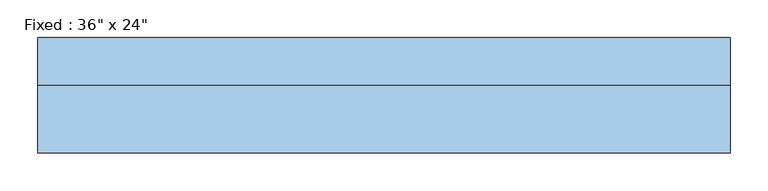
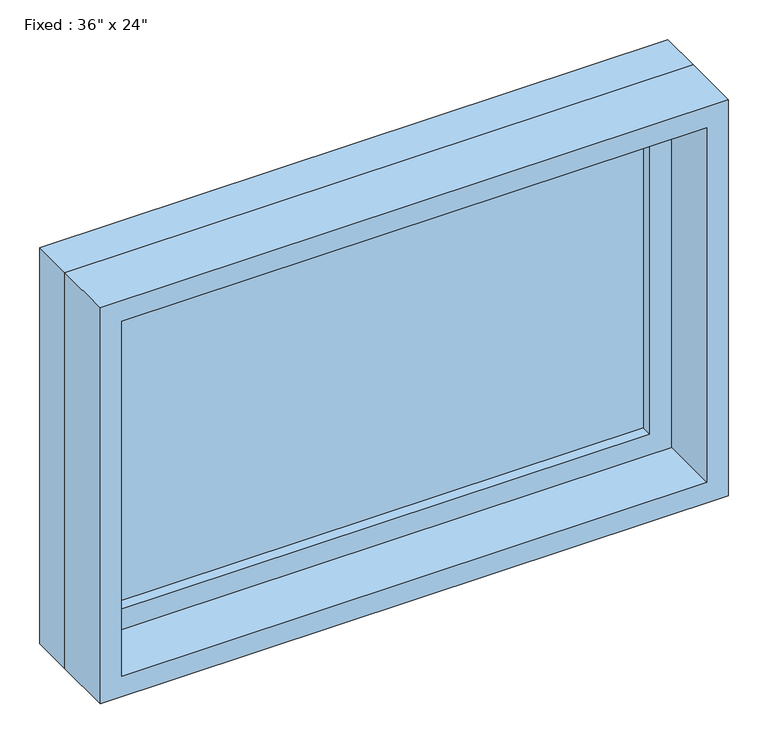
"""IFC4 building model written with IfcOpenShell, lengths in millimetres: window geometry."""

from ifc_helpers import new_model, si_unit, frame, origin, place, context, project, spatial, polyline, outline, extrude, source, transform, mapped, element, save


def window_fef7ae9c(model_context):
    return source(origin(), model_context, "Body", "SweptSolid", [
        extrude(outline(polyline([(355.6, 28.575), (-431.8, 28.575), (-431.8, 41.275), (355.6, 41.275), (355.6, 28.575)])), frame((0.0, 0.0, 977.9), z_axis=(0.0, 0.0, 1.0), x_axis=(1.0, 0.0, 0.0)), (0.0, 0.0, 1.0), 482.6),
        extrude(outline(polyline([(1504.95, -476.25), (933.45, -476.25), (933.45, 400.05), (1504.95, 400.05), (1504.95, -476.25)]), holes=[polyline([(1460.5, -431.8), (1460.5, 355.6), (977.9, 355.6), (977.9, -431.8), (1460.5, -431.8)])]), frame((0.0, 12.7, 0.0), z_axis=(0.0, 1.0, 0.0), x_axis=(0.0, 0.0, 1.0)), (0.0, 0.0, 1.0), 44.45),
        extrude(outline(polyline([(1524.0, -495.3), (914.4, -495.3), (914.4, 419.1), (1524.0, 419.1), (1524.0, -495.3)]), holes=[polyline([(1492.25, -463.55), (1492.25, 387.35), (946.15, 387.35), (946.15, -463.55), (1492.25, -463.55)])]), frame((0.0, -76.2, 0.0), z_axis=(0.0, 1.0, 0.0), x_axis=(0.0, 0.0, 1.0)), (0.0, 0.0, 1.0), 88.9),
        extrude(outline(polyline([(1524.0, 419.1), (1524.0, -495.3), (914.4, -495.3), (914.4, 419.1), (1524.0, 419.1)]), holes=[polyline([(1504.95, 400.05), (933.45, 400.05), (933.45, -476.25), (1504.95, -476.25), (1504.95, 400.05)])]), frame((0.0, 12.7, 0.0), z_axis=(0.0, 1.0, 0.0), x_axis=(0.0, 0.0, 1.0)), (0.0, 0.0, 1.0), 63.5),
    ])


if __name__ == "__main__":
    model = new_model("IFC4")
    model_context = context("Model", 3, world=origin())
    ifc_project = project(units=[si_unit("LENGTHUNIT", "METRE", prefix="MILLI")], contexts=[model_context])
    site = spatial("IfcSite", under=ifc_project)
    building = spatial("IfcBuilding", under=site)
    placement = place(None, origin())
    window_shape = window_fef7ae9c(model_context)
    element("IfcWindow", 1, ObjectType="Fixed : 36\" x 24\"", at=placement, inside=building, context=model_context, shape_type="MappedRepresentation", body=[
        mapped(window_shape, transform((0.0, 0.0, 0.0), x_axis=(1.0, 0.0, 0.0), y_axis=(0.0, 1.0, 0.0), z_axis=(0.0, 0.0, 1.0))),
    ])
    save(model, "model.ifc")

# Revit data of these elements
# Type "Fixed : 36\" x 24\""
#   Type Mark = "8"
#   Construction Type Id = "GSP4R"
#   Assembly Code = "B2020100"
#   Analytic Construction = "1/8 in Pilkington single glazing"
#   Visual Light Transmittance = 0.9
#   Solar Heat Gain Coefficient = 0.78
#   Heat Transfer Coefficient (U) = 0.6496 BTU/(h·ft²·°F)
#   Height = 2' - 0"
#   Default Sill Height = 3' - 0"
#   Width = 3' - 0"
#   Window Inset = 0' - 0 3/4"
#   Define Thermal Properties by = 1
#   Glass Pane Material = Glass
#   Sash Material = Sash
#   Wall Closure = (empty or 0)
# Element 1 (IfcWindow, "Fixed : 36\" x 24\"")
#   Materials on its faces: "Sash", "Glass"
# Materials
#   "Glass": class "Glass", colour RGB 0 128 192, transparency 0.75, Description = "Soda Lime Glass", Cost = 0
#   "Sash": class "Wood", colour RGB 224 178 126, transparency 0
